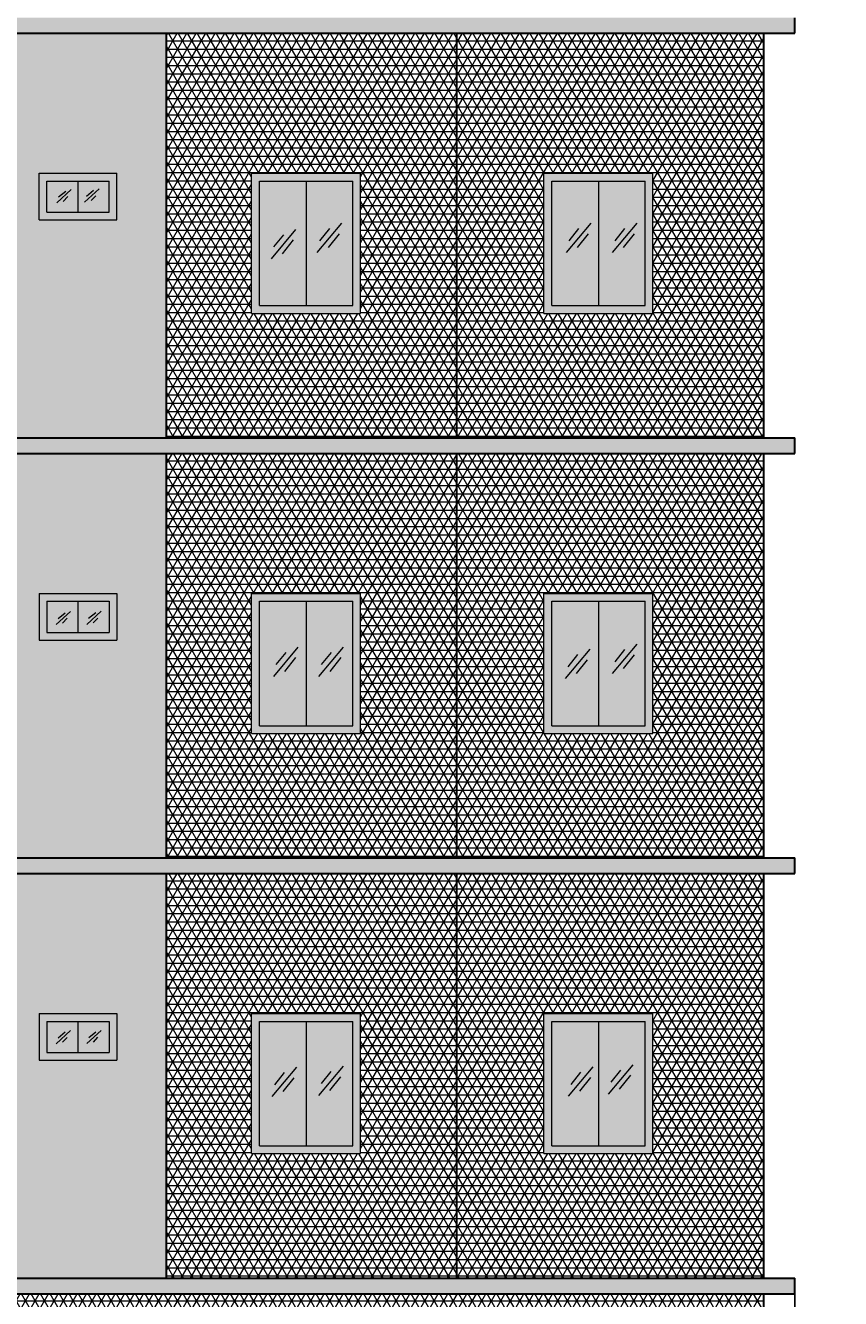
# Model space of a CAD drawing. Units: inches. Extents: x 2391 to 16591, y 7259 to 10239.
# Tile 9 of 27: x 3173 to 3487, y 7745 to 8236. Entities that reach past the tile are written whole.
import ezdxf

# ---------------------------------------------------------------- set-up
doc = ezdxf.new("R2010")
doc.units = ezdxf.units.IN
for name, color, linetype, lineweight in [('A-ANNO-DIMS', 4, 'Continuous', 18), ('A-ELEV', 7, 'Continuous', 30), ('A-ELEV-GLAZ', 4, 'Continuous', 18), ('A-ELEV-GLAZ-PATT', 141, 'Continuous', 13), ('A-ELEV-PATT', 8, 'Continuous', 13), ('A-ELEV-SURF-PATT', 253, 'Continuous', 13)]:
    doc.layers.add(name, color=color, linetype=linetype, lineweight=lineweight)
doc.styles.get("Standard").update_dxf_attribs({"font": 'arial.ttf'})
doc.dimstyles.new('ISO-25', dxfattribs={"dimtxt": 2.5, "dimasz": 2.5, "dimexe": 1.25, "dimexo": 0.625, "dimtad": 1, "dimdec": 0, "dimlunit": 3, "dimtxsty": 'Standard', "dimcen": 2.5, "dimadec": 0, "dimazin": 0, "dimtfac": 1, "dimtdec": 0, "dimtmove": 0, "dimatfit": 3, "dimfxl": 1, "dimarcsym": 0})

# ---------------------------------------------------------------- blocks, each defined once
blk = doc.blocks.new('GLASS-REFLECTION-VENT')
for p, q in [((0, 0), (5.55, 5.12)), ((0.7, 2.37), (3.45, 4.58)), ((2.48, 0.59), (4.26, 2.48))]:
    blk.add_line(p, q)
blk = doc.blocks.new('GLASS-REFLECTION-WINDOW')
for p, q in [((0, 0), (9.5, 11.3)), ((1, 4.52), (4.76, 9.26)), ((4.26, 1.91), (8.52, 7.21))]:
    blk.add_line(p, q)
blk = doc.blocks.new('*D83')
at = {"layer": 'A-ANNO-DIMS', "color": 0, "lineweight": -2, "transparency": 16777216}
for p, q in [((3013.78, 7751.89), (3013.78, 7528.22)), ((3469.78, 7751.89), (3469.78, 7528.22)), ((3016.28, 7529.47), (3467.28, 7529.47))]:
    blk.add_line(p, q, dxfattribs=at)
at = {"layer": 'A-ANNO-DIMS', "color": 0, "transparency": 16777216}
for points in [[(3016.28, 7529.89), (3016.28, 7529.05), (3013.78, 7529.47)], [(3467.28, 7529.89), (3467.28, 7529.05), (3469.78, 7529.47)]]:
    blk.add_solid(points, dxfattribs=at)
at = {"layer": 'Defpoints', "color": 0, "transparency": 16777216}
for p in [(3013.78, 7752.52), (3469.78, 7752.52), (3469.78, 7529.47)]:
    blk.add_point(p, dxfattribs=at)
at = {"layer": 'A-ANNO-DIMS', "color": 0, "transparency": 16777216, "insert": (3241.78, 7531.37), "char_height": 2.5, "attachment_point": 5}
blk.add_mtext('38\'-0"', dxfattribs=at)
blk = doc.blocks.new('*D84')
at = {"layer": 'A-ANNO-DIMS', "color": 0, "lineweight": -2, "transparency": 16777216}
for p, q in [((3437.4, 8339.52), (3518.08, 8339.52)), ((3516.83, 7579.02), (3516.83, 8337.02)), ((3464.4, 7576.52), (3518.08, 7576.52))]:
    blk.add_line(p, q, dxfattribs=at)
at = {"layer": 'A-ANNO-DIMS', "color": 0, "transparency": 16777216}
for points in [[(3516.41, 8337.02), (3517.24, 8337.02), (3516.83, 8339.52)], [(3516.41, 7579.02), (3517.24, 7579.02), (3516.83, 7576.52)]]:
    blk.add_solid(points, dxfattribs=at)
at = {"layer": 'Defpoints', "color": 0, "transparency": 16777216}
for p in [(3436.78, 8339.52), (3516.83, 8339.52), (3463.78, 7576.52)]:
    blk.add_point(p, dxfattribs=at)
at = {"layer": 'A-ANNO-DIMS', "color": 0, "transparency": 16777216, "insert": (3514.93, 7958.02), "char_height": 2.5, "attachment_point": 5, "rotation": 90}
blk.add_mtext('63\'-7"', dxfattribs=at)

msp = doc.modelspace()

# ---------------------------------------------------------------- hatches: boundary and pattern name
at = {"layer": 'A-ELEV-GLAZ-PATT'}
h = msp.add_hatch(color=256, dxfattribs=at)
h.dxf.hatch_style = 1
h.paths.add_polyline_path([(3208.28, 8178.52), (3178.28, 8178.52), (3178.28, 8160.52), (3208.28, 8160.52)])
h.paths.add_polyline_path([(3205.28, 8175.52), (3205.28, 8163.52), (3181.28, 8163.52), (3181.28, 8175.52)], flags=16)
h.paths.add_polyline_path([(3260.28, 8178.52), (3260.28, 8124.52), (3302.28, 8124.52), (3302.28, 8178.52)])
h.paths.add_polyline_path([(3299.28, 8175.52), (3299.28, 8127.52), (3263.28, 8127.52), (3263.28, 8175.52)], flags=16)
h.paths.add_polyline_path([(3415.03, 8178.52), (3373.03, 8178.52), (3373.03, 8124.52), (3415.03, 8124.52)])
h.paths.add_polyline_path([(3412.03, 8175.52), (3412.03, 8127.52), (3376.03, 8127.52), (3376.03, 8175.52)], flags=16)
h.paths.add_polyline_path([(3178.28, 8016.52), (3178.28, 7998.52), (3208.28, 7998.52), (3208.28, 8016.52)])
h.paths.add_polyline_path([(3205.28, 8013.52), (3205.28, 8001.52), (3181.28, 8001.52), (3181.28, 8013.52)], flags=16)
h.paths.add_polyline_path([(3260.28, 8016.52), (3260.28, 7962.52), (3302.28, 7962.52), (3302.28, 8016.52)])
h.paths.add_polyline_path([(3299.28, 8013.52), (3299.28, 7965.52), (3263.28, 7965.52), (3263.28, 8013.52)], flags=16)
h.paths.add_polyline_path([(3373.03, 8016.52), (3373.03, 7962.52), (3415.03, 7962.52), (3415.03, 8016.52)])
h.paths.add_polyline_path([(3376.03, 8013.52), (3412.03, 8013.52), (3412.03, 7965.52), (3376.03, 7965.52)], flags=16)
h.paths.add_polyline_path([(3208.28, 7854.52), (3178.28, 7854.52), (3178.28, 7836.52), (3208.28, 7836.52)])
h.paths.add_polyline_path([(3205.28, 7851.52), (3205.28, 7839.52), (3181.28, 7839.52), (3181.28, 7851.52)], flags=16)
h.paths.add_polyline_path([(3302.28, 7854.52), (3260.28, 7854.52), (3260.28, 7800.52), (3302.28, 7800.52)])
h.paths.add_polyline_path([(3263.28, 7851.52), (3299.28, 7851.52), (3299.28, 7803.52), (3263.28, 7803.52)], flags=16)
h.paths.add_polyline_path([(3373.03, 7854.52), (3373.03, 7800.52), (3415.03, 7800.52), (3415.03, 7854.52)])
h.paths.add_polyline_path([(3376.03, 7851.52), (3412.03, 7851.52), (3412.03, 7803.52), (3376.03, 7803.52)], flags=16)
h = msp.add_hatch(color=256, dxfattribs=at)
h.dxf.hatch_style = 1
h.paths.add_polyline_path([(3193.28, 8175.52), (3181.28, 8175.52), (3181.28, 8163.52), (3193.28, 8163.52)])
h.paths.add_polyline_path([(3205.28, 8175.52), (3193.28, 8175.52), (3193.28, 8163.52), (3205.28, 8163.52)])
h.paths.add_polyline_path([(3281.28, 8175.52), (3263.28, 8175.52), (3263.28, 8127.52), (3281.28, 8127.52)])
h.paths.add_polyline_path([(3299.28, 8175.52), (3281.28, 8175.52), (3281.28, 8127.52), (3299.28, 8127.52)])
h.paths.add_polyline_path([(3394.03, 8175.52), (3376.03, 8175.52), (3376.03, 8127.52), (3394.03, 8127.52)])
h.paths.add_polyline_path([(3412.03, 8175.52), (3394.03, 8175.52), (3394.03, 8127.52), (3412.03, 8127.52)])
h.paths.add_polyline_path([(3193.28, 8013.52), (3181.28, 8013.52), (3181.28, 8001.52), (3193.28, 8001.52)])
h.paths.add_polyline_path([(3205.28, 8013.52), (3193.28, 8013.52), (3193.28, 8001.52), (3205.28, 8001.52)])
h.paths.add_polyline_path([(3281.28, 8013.52), (3263.28, 8013.52), (3263.28, 7965.52), (3281.28, 7965.52)])
h.paths.add_polyline_path([(3299.28, 8013.52), (3281.28, 8013.52), (3281.28, 7965.52), (3299.28, 7965.52)])
h.paths.add_polyline_path([(3394.03, 8013.52), (3376.03, 8013.52), (3376.03, 7965.52), (3394.03, 7965.52)])
h.paths.add_polyline_path([(3412.03, 8013.52), (3394.03, 8013.52), (3394.03, 7965.52), (3412.03, 7965.52)])
h.paths.add_polyline_path([(3193.28, 7851.52), (3181.28, 7851.52), (3181.28, 7839.52), (3193.28, 7839.52)])
h.paths.add_polyline_path([(3205.28, 7851.52), (3193.28, 7851.52), (3193.28, 7839.52), (3205.28, 7839.52)])
h.paths.add_polyline_path([(3281.28, 7851.52), (3263.28, 7851.52), (3263.28, 7803.52), (3281.28, 7803.52)])
h.paths.add_polyline_path([(3299.28, 7851.52), (3281.28, 7851.52), (3281.28, 7803.52), (3299.28, 7803.52)])
h.paths.add_polyline_path([(3394.03, 7851.52), (3376.03, 7851.52), (3376.03, 7803.52), (3394.03, 7803.52)])
h.paths.add_polyline_path([(3412.03, 7851.52), (3394.03, 7851.52), (3394.03, 7803.52), (3412.03, 7803.52)])
at = {"layer": 'A-ELEV-PATT'}
h = msp.add_hatch(dxfattribs=at)
h.set_pattern_fill('NET3', color=256)
h.paths.add_polyline_path([(3457.78, 8232.52), (3339.28, 8232.52), (3339.28, 8076.52), (3457.78, 8076.52)])
h.paths.add_polyline_path([(3415.03, 8124.52), (3373.03, 8124.52), (3373.03, 8178.52), (3415.03, 8178.52)], flags=16)
h.paths.add_polyline_path([(3412.03, 8127.52), (3376.03, 8127.52), (3376.03, 8175.52), (3412.03, 8175.52)], flags=0)
h.paths.add_polyline_path([(3457.78, 8070.52), (3339.28, 8070.52), (3339.28, 7914.52), (3457.78, 7914.52)])
h.paths.add_polyline_path([(3415.03, 7962.52), (3373.03, 7962.52), (3373.03, 8016.52), (3415.03, 8016.52)], flags=16)
h.paths.add_polyline_path([(3412.03, 7965.52), (3376.03, 7965.52), (3376.03, 8013.52), (3412.03, 8013.52)], flags=0)
h.paths.add_polyline_path([(3457.78, 7908.52), (3339.28, 7908.52), (3339.28, 7752.52), (3457.78, 7752.52)])
h.paths.add_polyline_path([(3415.03, 7800.52), (3373.03, 7800.52), (3373.03, 7854.52), (3415.03, 7854.52)], flags=16)
h.paths.add_polyline_path([(3412.03, 7803.52), (3376.03, 7803.52), (3376.03, 7851.52), (3412.03, 7851.52)], flags=0)
h.paths.add_polyline_path([(3339.28, 8232.52), (3227.28, 8232.52), (3227.28, 8076.52), (3339.28, 8076.52)])
h.paths.add_polyline_path([(3260.28, 8124.52), (3260.28, 8178.52), (3302.28, 8178.52), (3302.28, 8124.52)], flags=16)
h.paths.add_polyline_path([(3263.28, 8127.52), (3263.28, 8175.52), (3299.28, 8175.52), (3299.28, 8127.52)], flags=0)
h.paths.add_polyline_path([(3339.28, 8070.52), (3227.28, 8070.52), (3227.28, 7914.52), (3339.28, 7914.52)])
h.paths.add_polyline_path([(3260.28, 8016.52), (3302.28, 8016.52), (3302.28, 7962.52), (3260.28, 7962.52)], flags=16)
h.paths.add_polyline_path([(3263.28, 8013.52), (3299.28, 8013.52), (3299.28, 7965.52), (3263.28, 7965.52)], flags=0)
h.paths.add_polyline_path([(3339.28, 7908.52), (3227.28, 7908.52), (3227.28, 7752.52), (3339.28, 7752.52)])
h.paths.add_polyline_path([(3260.28, 7854.52), (3302.28, 7854.52), (3302.28, 7800.52), (3260.28, 7800.52)], flags=16)
h.paths.add_polyline_path([(3263.28, 7851.52), (3299.28, 7851.52), (3299.28, 7803.52), (3263.28, 7803.52)], flags=0)
h.paths.add_polyline_path([(3213.78, 7717.52), (3232.78, 7717.52), (3232.78, 7712.52), (3227.78, 7712.52), (3227.78, 7683.36), (3230.28, 7683.36), (3230.28, 7685.36), (3232.78, 7685.36), (3232.78, 7710.52), (3301.78, 7710.52), (3301.78, 7595.52), (3232.78, 7595.52), (3232.78, 7590.52), (3371.78, 7590.52), (3371.78, 7595.52), (3302.78, 7595.52), (3302.78, 7710.52), (3371.78, 7710.52), (3371.78, 7685.36), (3374.28, 7685.36), (3374.28, 7683.36), (3376.78, 7683.36), (3376.78, 7712.52), (3371.78, 7712.52), (3371.78, 7717.52), (3390.78, 7717.52), (3390.78, 7712.52), (3385.78, 7712.52), (3385.78, 7703.52), (3457.78, 7703.52), (3457.78, 7746.52), (3025.78, 7746.52), (3025.78, 7703.52), (3218.78, 7703.52), (3218.78, 7712.52), (3213.78, 7712.52)])
h.paths.add_polyline_path([(3232.78, 7679.36), (3230.28, 7679.36), (3230.28, 7681.36), (3227.78, 7681.36), (3227.78, 7623.23), (3230.28, 7623.23), (3230.28, 7625.23), (3232.78, 7625.23)], flags=17)
h.paths.add_polyline_path([(3232.78, 7619.23), (3230.28, 7619.23), (3230.28, 7621.23), (3227.78, 7621.23), (3227.78, 7590.52), (3232.78, 7590.52)], flags=17)
h.paths.add_polyline_path([(3376.78, 7681.36), (3374.28, 7681.36), (3374.28, 7679.36), (3371.78, 7679.36), (3371.78, 7625.23), (3374.28, 7625.23), (3374.28, 7623.23), (3376.78, 7623.23)], flags=17)
h.paths.add_polyline_path([(3376.78, 7621.23), (3374.28, 7621.23), (3374.28, 7619.23), (3371.78, 7619.23), (3371.78, 7590.52), (3376.78, 7590.52)], flags=17)
h = msp.add_hatch(dxfattribs=at)
h.set_pattern_fill('SQUARE', color=256)
h.paths.add_polyline_path([(3227.28, 8076.52), (3227.28, 8232.52), (3025.78, 8232.52), (3025.78, 8076.52)])
h.paths.add_polyline_path([(3178.28, 8160.52), (3178.28, 8178.52), (3208.28, 8178.52), (3208.28, 8160.52)], flags=16)
h.paths.add_polyline_path([(3181.28, 8163.52), (3181.28, 8175.52), (3205.28, 8175.52), (3205.28, 8163.52)], flags=0)
h.paths.add_polyline_path([(3025.78, 8070.52), (3025.78, 7914.52), (3227.28, 7914.52), (3227.28, 8070.52)])
h.paths.add_polyline_path([(3178.28, 7998.52), (3178.28, 8016.52), (3208.28, 8016.52), (3208.28, 7998.52)], flags=16)
h.paths.add_polyline_path([(3181.28, 8001.52), (3181.28, 8013.52), (3205.28, 8013.52), (3205.28, 8001.52)], flags=0)
h.paths.add_polyline_path([(3025.78, 7908.52), (3025.78, 7752.52), (3227.28, 7752.52), (3227.28, 7908.52)])
h.paths.add_polyline_path([(3178.28, 7854.52), (3208.28, 7854.52), (3208.28, 7836.52), (3178.28, 7836.52)], flags=16)
h.paths.add_polyline_path([(3181.28, 7851.52), (3205.28, 7851.52), (3205.28, 7839.52), (3181.28, 7839.52)], flags=0)
at = {"layer": 'A-ELEV-SURF-PATT'}
h = msp.add_hatch(color=256, dxfattribs=at)
h.dxf.hatch_style = 1
h.paths.add_polyline_path([(3469.78, 7746.52), (3469.78, 7752.52), (3013.78, 7752.52), (3013.78, 7746.52)])
h.paths.add_polyline_path([(3469.78, 7908.52), (3469.78, 7914.52), (3013.78, 7914.52), (3013.78, 7908.52)])
h.paths.add_polyline_path([(3469.78, 8070.52), (3469.78, 8076.52), (3013.78, 8076.52), (3013.78, 8070.52)])
h.paths.add_polyline_path([(3013.78, 8238.52), (3013.78, 8232.52), (3469.78, 8232.52), (3469.78, 8238.52)])
h.paths.add_polyline_path([(3236.28, 8339.52), (3236.28, 8334.52), (3436.78, 8334.52), (3436.78, 8339.52)])

# ---------------------------------------------------------------- linework, layer by layer
at = {"layer": 'A-ELEV'}
for p, q in [((3469.78, 8232.52), (3469.78, 8238.52)), ((3013.78, 8232.52), (3469.78, 8232.52)), ((3227.28, 8232.52), (3227.28, 8076.52)), ((3339.28, 8232.52), (3339.28, 8076.52)), ((3457.78, 8076.52), (3457.78, 8232.52)), ((3013.78, 8076.52), (3469.78, 8076.52)), ((3469.78, 8070.52), (3469.78, 8076.52)), ((3013.78, 8070.52), (3469.78, 8070.52)), ((3227.28, 8070.52), (3227.28, 7914.52)), ((3339.28, 8070.52), (3339.28, 7914.52)), ((3457.78, 7914.52), (3457.78, 8070.52)), ((3013.78, 7914.52), (3469.78, 7914.52)), ((3469.78, 7908.52), (3469.78, 7914.52)), ((3013.78, 7908.52), (3469.78, 7908.52)), ((3227.28, 7908.52), (3227.28, 7752.52)), ((3339.28, 7908.52), (3339.28, 7752.52)), ((3457.78, 7752.52), (3457.78, 7908.52)), ((3013.78, 7752.52), (3469.78, 7752.52)), ((3469.78, 7746.52), (3469.78, 7752.52)), ((3013.78, 7746.52), (3469.78, 7746.52)), ((3457.78, 7581.52), (3457.78, 7746.52))]:
    msp.add_line(p, q, dxfattribs=at)
at = {"layer": 'A-ELEV-GLAZ'}
for p, q in [((3178.28, 8178.52), (3208.28, 8178.52)), ((3178.28, 8160.52), (3178.28, 8178.52)), ((3208.28, 8160.52), (3208.28, 8178.52)), ((3260.28, 8178.52), (3302.28, 8178.52)), ((3260.28, 8124.52), (3260.28, 8178.52)), ((3302.28, 8124.52), (3302.28, 8178.52)), ((3373.03, 8178.52), (3415.03, 8178.52)), ((3373.03, 8124.52), (3373.03, 8178.52)), ((3415.03, 8124.52), (3415.03, 8178.52)), ((3181.28, 8175.52), (3205.28, 8175.52)), ((3181.28, 8163.52), (3181.28, 8175.52)), ((3193.28, 8175.52), (3193.28, 8163.52)), ((3205.28, 8163.52), (3205.28, 8175.52)), ((3263.28, 8175.52), (3299.28, 8175.52)), ((3263.28, 8127.52), (3263.28, 8175.52)), ((3281.28, 8175.52), (3281.28, 8127.52)), ((3299.28, 8127.52), (3299.28, 8175.52)), ((3376.03, 8175.52), (3412.03, 8175.52)), ((3376.03, 8127.52), (3376.03, 8175.52)), ((3394.03, 8175.52), (3394.03, 8127.52)), ((3412.03, 8127.52), (3412.03, 8175.52)), ((3181.28, 8163.52), (3205.28, 8163.52)), ((3178.28, 8160.52), (3208.28, 8160.52)), ((3260.28, 8124.52), (3302.28, 8124.52)), ((3263.28, 8127.52), (3299.28, 8127.52)), ((3373.03, 8124.52), (3415.03, 8124.52)), ((3376.03, 8127.52), (3412.03, 8127.52)), ((3178.28, 8016.52), (3208.28, 8016.52)), ((3178.28, 8016.52), (3178.28, 7998.52)), ((3208.28, 8016.52), (3208.28, 7998.52)), ((3260.28, 8016.52), (3302.28, 8016.52)), ((3260.28, 7962.52), (3260.28, 8016.52)), ((3302.28, 7962.52), (3302.28, 8016.52)), ((3373.03, 8016.52), (3415.03, 8016.52)), ((3373.03, 7962.52), (3373.03, 8016.52)), ((3415.03, 7962.52), (3415.03, 8016.52)), ((3181.28, 8013.52), (3205.28, 8013.52)), ((3181.28, 8013.52), (3181.28, 8001.52)), ((3193.28, 8013.52), (3193.28, 8001.52)), ((3205.28, 8013.52), (3205.28, 8001.52)), ((3263.28, 8013.52), (3299.28, 8013.52)), ((3263.28, 7965.52), (3263.28, 8013.52)), ((3281.28, 8013.52), (3281.28, 7965.52)), ((3299.28, 7965.52), (3299.28, 8013.52)), ((3376.03, 8013.52), (3412.03, 8013.52)), ((3376.03, 7965.52), (3376.03, 8013.52)), ((3394.03, 8013.52), (3394.03, 7965.52)), ((3412.03, 7965.52), (3412.03, 8013.52)), ((3181.28, 8001.52), (3205.28, 8001.52)), ((3178.28, 7998.52), (3208.28, 7998.52)), ((3260.28, 7962.52), (3302.28, 7962.52)), ((3263.28, 7965.52), (3299.28, 7965.52)), ((3373.03, 7962.52), (3415.03, 7962.52)), ((3376.03, 7965.52), (3412.03, 7965.52)), ((3178.28, 7854.52), (3208.28, 7854.52)), ((3178.28, 7854.52), (3178.28, 7836.52)), ((3208.28, 7854.52), (3208.28, 7836.52)), ((3260.28, 7854.52), (3302.28, 7854.52)), ((3260.28, 7800.52), (3260.28, 7854.52)), ((3302.28, 7800.52), (3302.28, 7854.52)), ((3373.03, 7854.52), (3415.03, 7854.52)), ((3373.03, 7800.52), (3373.03, 7854.52)), ((3415.03, 7800.52), (3415.03, 7854.52)), ((3181.28, 7851.52), (3205.28, 7851.52)), ((3181.28, 7851.52), (3181.28, 7839.52)), ((3193.28, 7851.52), (3193.28, 7839.52)), ((3205.28, 7851.52), (3205.28, 7839.52)), ((3263.28, 7851.52), (3299.28, 7851.52)), ((3263.28, 7803.52), (3263.28, 7851.52)), ((3281.28, 7851.52), (3281.28, 7803.52)), ((3299.28, 7803.52), (3299.28, 7851.52)), ((3376.03, 7851.52), (3412.03, 7851.52)), ((3376.03, 7803.52), (3376.03, 7851.52)), ((3394.03, 7851.52), (3394.03, 7803.52)), ((3412.03, 7803.52), (3412.03, 7851.52)), ((3181.28, 7839.52), (3205.28, 7839.52)), ((3178.28, 7836.52), (3208.28, 7836.52)), ((3260.28, 7800.52), (3302.28, 7800.52)), ((3263.28, 7803.52), (3299.28, 7803.52)), ((3373.03, 7800.52), (3415.03, 7800.52)), ((3376.03, 7803.52), (3412.03, 7803.52))]:
    msp.add_line(p, q, dxfattribs=at)

# ---------------------------------------------------------------- block references
for name, p in [('GLASS-REFLECTION-VENT', (3185.11, 8167.1)), ('GLASS-REFLECTION-VENT', (3195.86, 8167.38)), ('GLASS-REFLECTION-WINDOW', (3285.61, 8147.94)), ('GLASS-REFLECTION-WINDOW', (3381.72, 8147.94)), ('GLASS-REFLECTION-WINDOW', (3399.44, 8147.94)), ('GLASS-REFLECTION-WINDOW', (3267.88, 8145.59)), ('GLASS-REFLECTION-VENT', (3184.89, 8004.49)), ('GLASS-REFLECTION-VENT', (3196.67, 8004.56)), ('GLASS-REFLECTION-WINDOW', (3399.44, 7985.62)), ('GLASS-REFLECTION-WINDOW', (3268.78, 7984.55)), ('GLASS-REFLECTION-WINDOW', (3286.25, 7984.55)), ('GLASS-REFLECTION-WINDOW', (3381.33, 7983.71)), ('GLASS-REFLECTION-VENT', (3184.89, 7842.87)), ('GLASS-REFLECTION-VENT', (3196.75, 7842.93)), ('GLASS-REFLECTION-WINDOW', (3286.2, 7822.99)), ('GLASS-REFLECTION-WINDOW', (3397.95, 7823.51)), ('GLASS-REFLECTION-WINDOW', (3268.17, 7822.57)), ('GLASS-REFLECTION-WINDOW', (3382.53, 7822.72))]:
    msp.add_blockref(name, p, dxfattribs=at)

# ---------------------------------------------------------------- dimensions: what is measured, and where the dimension line sits
at = {"layer": 'A-ANNO-DIMS'}
dim = msp.add_linear_dim(base=(3516.83, 8339.52), p1=(3463.78, 7576.52), p2=(3436.78, 8339.52), angle=90, dimstyle='ISO-25', override={"dimdec": 1, "dimlfac": 1, "dimrnd": 0, "dimzin": 1, "dimdsep": 46, "dimlunit": 4, "dimfrac": 2}, dxfattribs=at)
dim.commit()
dim.dimension.update_dxf_attribs({"geometry": '*D84', "text_midpoint": (3514.93, 7958.02)})
dim = msp.add_linear_dim(base=(3469.78, 7529.47), p1=(3013.78, 7752.52), p2=(3469.78, 7752.52), dimstyle='ISO-25', override={"dimdec": 1, "dimlfac": 1, "dimrnd": 0, "dimzin": 1, "dimdsep": 46, "dimlunit": 4, "dimfrac": 2}, dxfattribs=at)
dim.commit()
dim.dimension.update_dxf_attribs({"geometry": '*D83', "text_midpoint": (3241.78, 7531.37)})

doc.saveas('drawing.dxf')
